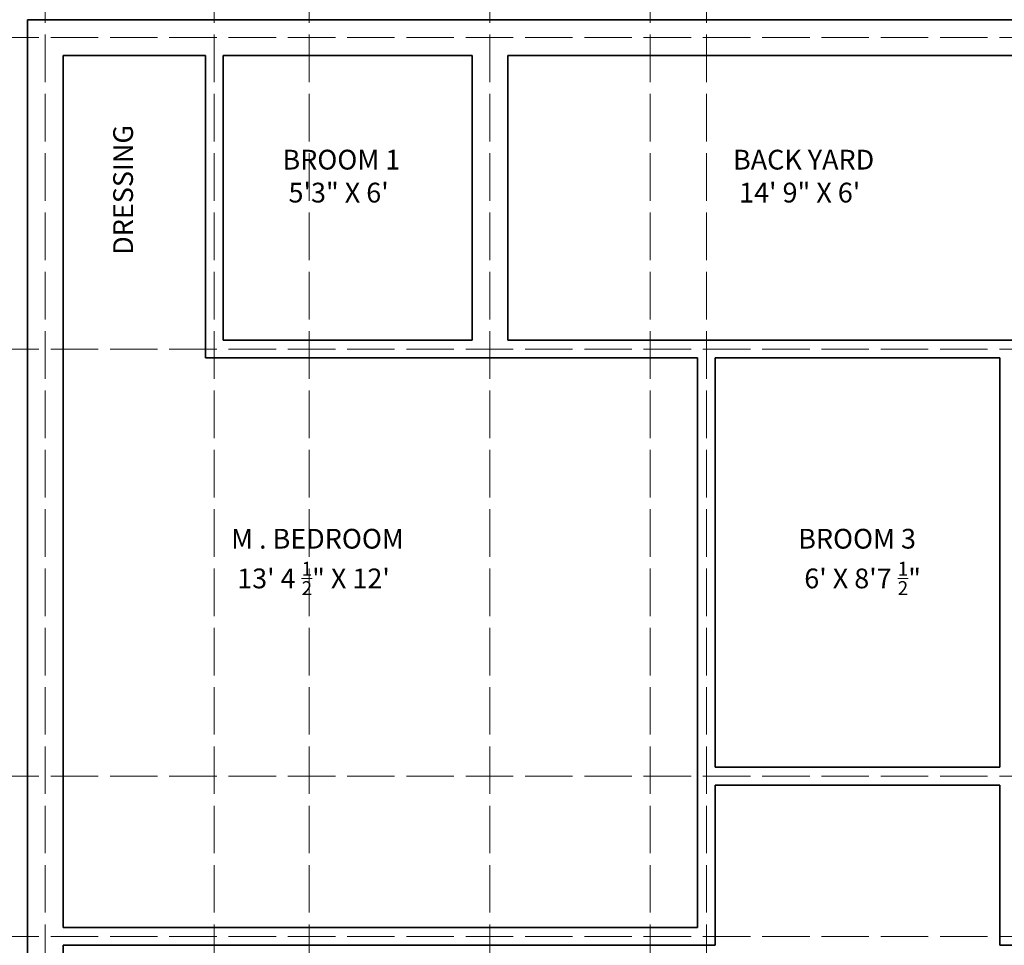
# Model space of a CAD drawing. Units: inches. Extents: x 1159 to 4240, y 1112 to 2085.
# Tile 6 of 13: x 1286 to 1535, y 1734 to 1968. Entities that reach past the tile are written whole.
import ezdxf

# ---------------------------------------------------------------- set-up
doc = ezdxf.new("R2010")
doc.units = ezdxf.units.IN
doc.linetypes.add('ACAD_ISO02W100', pattern=[15, 12, -3])
for name, color, linetype, lineweight in [('A-AREA-IDEN', 30, 'Continuous', 18), ('A-GRID', 8, 'ACAD_ISO02W100', 13), ('WALL', 7, 'Continuous', 35)]:
    doc.layers.add(name, color=color, linetype=linetype, lineweight=lineweight)
doc.styles.get("Standard").update_dxf_attribs({"font": 'arial.ttf'})

# ---------------------------------------------------------------- blocks, each defined once
blk = doc.blocks.new('HOUSE-35x60-WALL-LAYOUT')
for p, q in [((0, 0), (0, 720)), ((0, 720), (420, 720)), ((9, 711), (45, 711)), ((9, 634.5), (9, 711)), ((45, 634.5), (45, 711)), ((49.5, 639), (49.5, 711)), ((49.5, 711), (112.5, 711)), ((112.5, 639), (112.5, 711)), ((121.5, 639), (121.5, 711)), ((121.5, 711), (298.5, 711)), ((49.5, 639), (112.5, 639)), ((121.5, 639), (298.5, 639)), ((9, 490.5), (9, 634.5)), ((45, 634.5), (169.5, 634.5)), ((169.5, 634.5), (169.5, 490.5)), ((174, 634.5), (174, 531)), ((174, 634.5), (246, 634.5)), ((246, 634.5), (246, 531)), ((174, 531), (246, 531)), ((174, 526.5), (246, 526.5)), ((174, 526.5), (174, 486)), ((246, 526.5), (246, 486)), ((9, 490.5), (169.5, 490.5)), ((9, 486), (174, 486)), ((9, 306), (9, 486)), ((246, 486), (286.5, 486))]:
    blk.add_line(p, q)
blk = doc.blocks.new('HOUSE-35x60-SETTING-OUT-GRID')
for p, q in [((89.32, 0), (89.32, 883.25)), ((132.07, 0), (132.07, 883.25)), ((156.07, 0), (156.07, 883.25)), ((201.82, 0), (201.82, 883.25)), ((242.32, 0), (242.32, 883.25)), ((256.57, 0), (256.57, 883.25)), ((582.7, 806.25), (0, 806.25)), ((582.7, 727.5), (0, 727.5)), ((582.7, 619.5), (0, 619.5)), ((582.7, 579), (0, 579))]:
    blk.add_line(p, q)

msp = doc.modelspace()

# ---------------------------------------------------------------- block references
at = {"layer": 'A-GRID'}
msp.add_blockref('HOUSE-35x60-SETTING-OUT-GRID', (1203.31, 1156.954), dxfattribs=at)
at = {"layer": 'WALL'}
msp.add_blockref('HOUSE-35x60-WALL-LAYOUT', (1288.126, 1247.702), dxfattribs=at)

# ---------------------------------------------------------------- texts
at = {"layer": 'A-AREA-IDEN', "insert": (1309.814, 1908.276), "char_height": 5, "attachment_point": 1, "rotation": 90}
msp.add_mtext_dynamic_manual_height_columns('\\A1;DRESSING', width=140.18614, gutter_width=12.5, heights=[0], dxfattribs=at)
at = {"layer": 'A-AREA-IDEN', "char_height": 5, "attachment_point": 1}
for s, insert in [('\\A1;BROOM 1\\P 5\'3" X 6\'', (1352.638, 1934.831)), ('\\A1;BACK YARD\\P 14\' 9" X 6\'', (1466.625, 1934.831)), ('\\A1;M . BEDROOM\\P 13\' 4 {\\H0.7x;\\S1/2;}" X 12\'', (1339.649, 1838.992)), ('\\A1;BROOM 3\\P 6\' X 8\'7 {\\H0.7x;\\S1/2;}"', (1483.116, 1838.992))]:
    msp.add_mtext_dynamic_manual_height_columns(s, width=140.18614, gutter_width=12.5, heights=[0], dxfattribs=dict(at, insert=insert))

doc.saveas('drawing.dxf')
